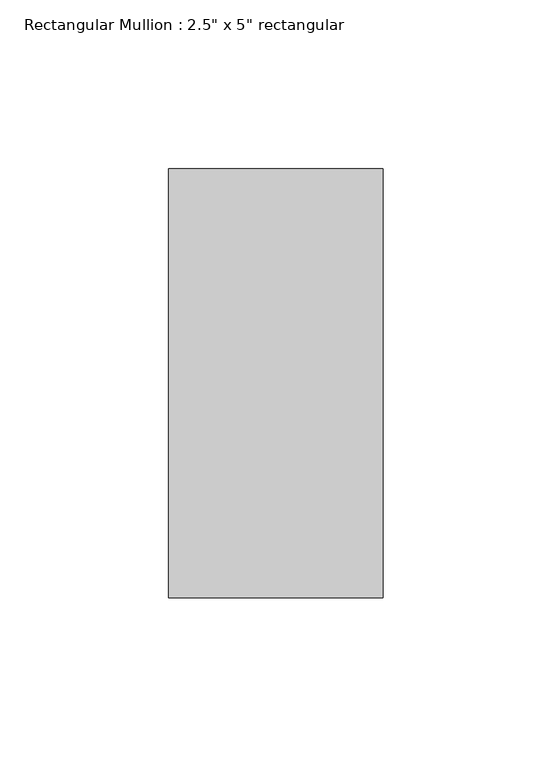
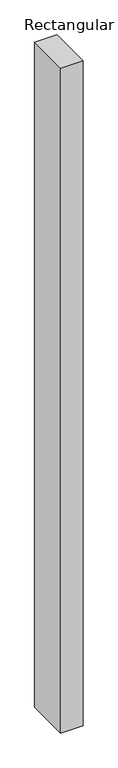
"""IFC4 building model written with IfcOpenShell, lengths in millimetres: member geometry."""

from ifc_helpers import new_model, si_unit, frame, origin, place, context, project, spatial, polyline, outline, extrude, source, transform, mapped, element, save


def member_bb8a6b57(model_context):
    return source(origin(), model_context, "Body", "SweptSolid", [
        extrude(outline(polyline([(0.0, 63.5), (0.0, -63.5), (-63.5, -63.5), (-63.5, 63.5), (0.0, 63.5)])), frame((0.0, 0.0, -1988.3028629), z_axis=(0.0, 0.0, 1.0), x_axis=(1.0, 0.0, 0.0)), (0.0, 0.0, 1.0), 1988.3028629),
    ])


if __name__ == "__main__":
    model = new_model("IFC4")
    model_context = context("Model", 3, world=origin())
    ifc_project = project(units=[si_unit("LENGTHUNIT", "METRE", prefix="MILLI")], contexts=[model_context])
    site = spatial("IfcSite", under=ifc_project)
    building = spatial("IfcBuilding", under=site)
    placement = place(None, origin())
    member_shape = member_bb8a6b57(model_context)
    element("IfcMember", 1, ObjectType="Rectangular Mullion : 2.5\" x 5\" rectangular", at=placement, inside=building, context=model_context, shape_type="MappedRepresentation", body=[
        mapped(member_shape, transform((0.0, 0.0, 0.0), x_axis=(1.0, 0.0, 0.0), y_axis=(0.0, 1.0, 0.0), z_axis=(0.0, 0.0, 1.0))),
    ])
    save(model, "model.ifc")

# Revit data of these elements
# Type "Rectangular Mullion : 2.5\" x 5\" rectangular"
#   built-in parameter 1007304 = 0.416667 (stored number, unit not read)
#   built-in parameter 1007301 = 0.104167 (stored number, unit not read)
#   built-in parameter 1007300 = 0.104167 (stored number, unit not read)
# Element 1 (IfcMember, "Rectangular Mullion : 2.5\" x 5\" rectangular")
#   Materials on its faces: "Aluminum"
# Materials
#   "Aluminum": class "Metal", colour RGB 247 247 247, transparency 0, Description = "Aluminum 6061", Cost = 0
